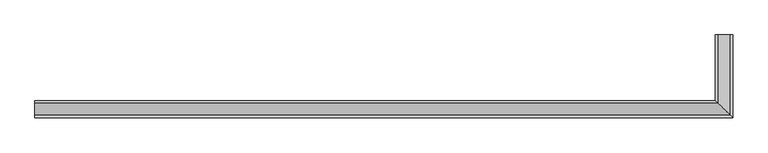
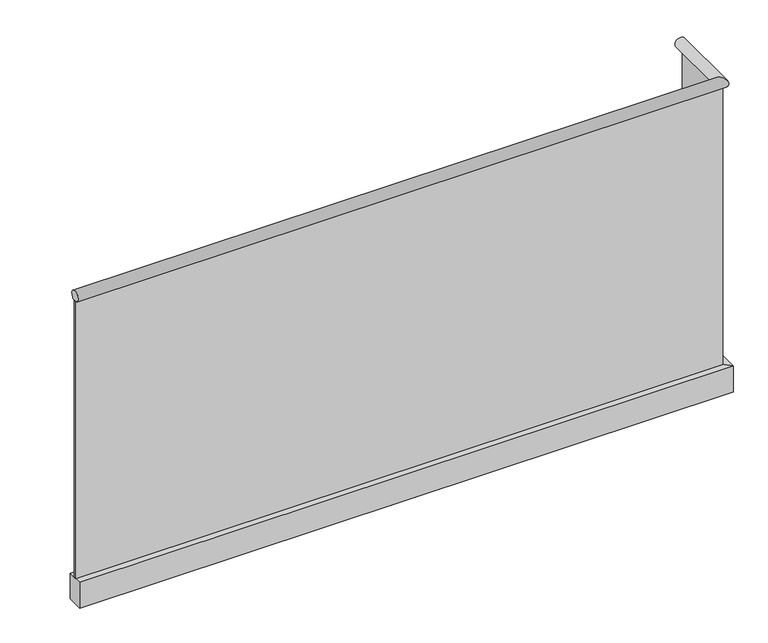
"""IFC4 building model written with IfcOpenShell, lengths in millimetres: railing geometry."""

from ifc_helpers import new_model, si_unit, frame, origin, place, context, project, spatial, circle_curve, ellipse_curve, faceted_brep, source, transform, mapped, element, save
from ifc_brep_helpers import plane_surface, cylinder_surface, advanced_brep


def railing_84ac703c(model_context):
    return source(origin(), model_context, "Body", "SolidModel", [
        advanced_brep(
        [(-5348.8712297, -8202.0014262, 4998.0), (-5348.8712297, -8182.0014262, 4998.0), (-2923.8712297, -8202.0014262, 4998.0), (-2943.8712297, -8182.0014262, 4998.0), (-2923.8712297, -7932.0014262, 4998.0), (-2943.8712297, -7932.0014262, 4998.0)],
        [
            (0, 1, circle_curve(frame((-5348.8712297, -8192.0014262, 5015.3205081), z_axis=(-1.0, 0.0, 0.0), x_axis=(0.0, -1.0, 0.0)), 20.0)),
            (1, 0),
            (0, 2),
            (2, 3, ellipse_curve(frame((-2933.8712297, -8192.0014262, 5015.3205081), z_axis=(-0.7071067811865496, -0.7071067811865455, 0.0), x_axis=(-0.7071067811865454, 0.7071067811865496, 0.0)), 28.2842712, 20.0)),
            (3, 1),
            (3, 2),
            (4, 5),
            (5, 4, circle_curve(frame((-2933.8712297, -7932.0014262, 5015.3205081), z_axis=(0.0, 1.0, 0.0), x_axis=(1.0, 0.0, 0.0)), 20.0)),
            (2, 4),
            (5, 3),
        ],
        [
            plane_surface(frame((-5348.8712297, -8192.0014262, 4998.0), z_axis=(-1.0, 0.0, 0.0), x_axis=(0.0, 1.0, 0.0))),
            cylinder_surface(frame((-5348.8712297, -8192.0014262, 5015.3205081), z_axis=(-1.0, 0.0, 0.0), x_axis=(0.0, -1.0, 0.0)), 20.0),
            plane_surface(frame((-5348.8712297, -8182.0014262, 4998.0), z_axis=(0.0, 0.0, -1.0), x_axis=(1.0, 0.0, 0.0))),
            plane_surface(frame((-2933.8712297, -7932.0014262, 4998.0), z_axis=(0.0, 1.0, 0.0), x_axis=(0.0, 0.0, 1.0))),
            cylinder_surface(frame((-2933.8712297, -8192.0014262, 5015.3205081), z_axis=(0.0, -1.0, 0.0), x_axis=(1.0, 0.0, 0.0)), 20.0),
            plane_surface(frame((-2943.8712297, -8182.0014262, 4998.0), z_axis=(0.0, 0.0, -1.0), x_axis=(0.0, 1.0, 0.0))),
        ],
        [
            (0, [[1, 2]]),
            (1, [[-1, 3, 4, 5]]),
            (2, [[-2, -5, 6, -3]]),
            (3, [[7, 8]]),
            (4, [[-4, 9, -8, 10]]),
            (5, [[-6, -10, -7, -9]]),
        ],
    ),
        faceted_brep([(-5348.8712297, -8198.0014262, 4998.0), (-5348.8712297, -8186.0014262, 4998.0), (-5348.8712297, -8186.0014262, 3900.0), (-5348.8712297, -8198.0014262, 3900.0), (-2927.8712297, -8198.0014262, 4998.0), (-2939.8712297, -8186.0014262, 4998.0), (-2939.8712297, -8186.0014262, 3900.0), (-2927.8712297, -8198.0014262, 3900.0), (-2927.8712297, -7968.0014262, 4998.0), (-2939.8712297, -7956.0014262, 4998.0), (-2939.8712297, -7956.0014262, 3900.0), (-2927.8712297, -7968.0014262, 3900.0), (-2923.8712297, -7968.0014262, 4998.0), (-2923.8712297, -7968.0014262, 3900.0), (-2923.8712297, -7956.0014262, 3900.0), (-2923.8712297, -7956.0014262, 4998.0)], [[[0, 1, 2, 3]], [[1, 0, 4, 5]], [[2, 1, 5, 6]], [[3, 2, 6, 7]], [[0, 3, 7, 4]], [[5, 4, 8, 9]], [[6, 5, 9, 10]], [[7, 6, 10, 11]], [[4, 7, 11, 8]], [[12, 13, 14, 15]], [[9, 8, 12, 15]], [[10, 9, 15, 14]], [[11, 10, 14, 13]], [[8, 11, 13, 12]]]),
        faceted_brep([(-5348.8712297, -8222.0014262, 3798.0), (-5348.8712297, -8222.0014262, 3900.0), (-5348.8712297, -8162.0014262, 3900.0), (-5348.8712297, -8162.0014262, 3798.0), (-2903.8712297, -8222.0014262, 3798.0), (-2903.8712297, -8222.0014262, 3900.0), (-2963.8712297, -8162.0014262, 3900.0), (-2963.8712297, -8162.0014262, 3798.0), (-2903.8712297, -7932.0014262, 3798.0), (-2963.8712297, -7932.0014262, 3798.0), (-2963.8712297, -7932.0014262, 3900.0), (-2903.8712297, -7932.0014262, 3900.0)], [[[0, 1, 2, 3]], [[1, 0, 4, 5]], [[2, 1, 5, 6]], [[3, 2, 6, 7]], [[0, 3, 7, 4]], [[8, 9, 10, 11]], [[5, 4, 8, 11]], [[6, 5, 11, 10]], [[7, 6, 10, 9]], [[4, 7, 9, 8]]]),
    ])


if __name__ == "__main__":
    model = new_model("IFC4")
    model_context = context("Model", 3, world=origin())
    ifc_project = project(units=[si_unit("LENGTHUNIT", "METRE", prefix="MILLI")], contexts=[model_context])
    site = spatial("IfcSite", under=ifc_project)
    building = spatial("IfcBuilding", under=site)
    placement = place(None, origin())
    railing_shape = railing_84ac703c(model_context)
    element("IfcRailing", 1, at=placement, inside=building, context=model_context, shape_type="MappedRepresentation", body=[
        mapped(railing_shape, transform((0.0, 0.0, 0.0), x_axis=(1.0, 0.0, 0.0), y_axis=(0.0, 1.0, 0.0), z_axis=(0.0, 0.0, 1.0))),
    ])
    save(model, "model.ifc")

# Revit data of these elements
# Element 1 (IfcRailing)
#   Materials on its faces: "Metal - Aluminum"
# Materials
#   "Metal - Aluminum": colour RGB 247 247 247, transparency 0, Cost = 0
